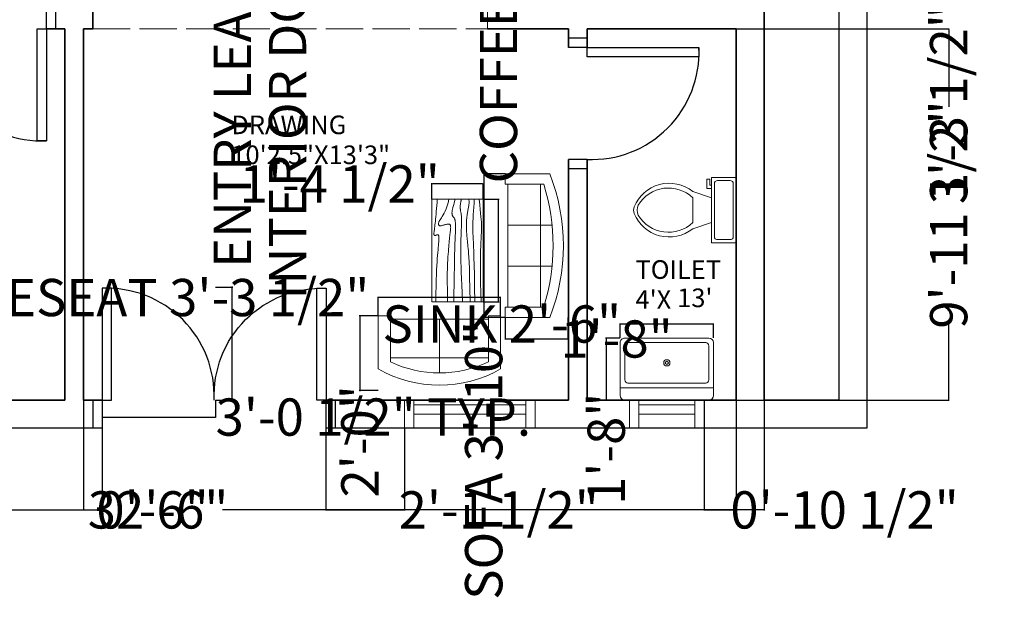
# Model space of a CAD drawing. Units: inches. Extents: x -107 to 531, y -526 to 131.
# Tile 2 of 4: x 205 to 522, y -526 to -340. Entities that reach past the tile are written whole.
import ezdxf

# ---------------------------------------------------------------- set-up
doc = ezdxf.new("R2010")
doc.units = ezdxf.units.IN
doc.header["$MEASUREMENT"] = 0
doc.linetypes.add('ACAD_ISO02W100', pattern=[15, 12, -3])
for name, color, linetype, lineweight in [('A-ANNO-DIMS', 2, 'Continuous', 18), ('A-AREA-IDEN', 7, 'Continuous', 25), ('A-DOOR', 3, 'Continuous', 25), ('A-FLOR-FIXT', 9, 'Continuous', 18), ('A-FLOR-STRS', 7, 'Continuous', 20), ('A-FURN', 8, 'Continuous', 18), ('A-GLAZ', 4, 'Continuous', 18), ('A-WALL', 7, 'Continuous', 35), ('A-WALL-OVHD', 8, 'ACAD_ISO02W100', 18), ('C-PROP', 8, 'Continuous', 25)]:
    doc.layers.add(name, color=color, linetype=linetype, lineweight=lineweight)
doc.styles.get("Standard").update_dxf_attribs({"font": 'arial.ttf'})
doc.dimstyles.get("Standard").update_dxf_attribs({"dimtxt": 12, "dimasz": 0.18, "dimexe": 0.18, "dimexo": 0.0625, "dimgap": 0.09, "dimtad": 0, "dimdec": 1, "dimzin": 0, "dimdsep": 46, "dimlunit": 3, "dimtxsty": 'Standard', "dimcen": 0.09, "dimadec": 0, "dimazin": 0, "dimtfac": 1, "dimtdec": 1, "dimtofl": 0, "dimtmove": 0, "dimatfit": 3, "dimfxl": 1, "dimtolj": 1, "dimtzin": 0, "dimarcsym": 0})

# ---------------------------------------------------------------- blocks, each defined once
blk = doc.blocks.new('Sofa - Roundback 7 ft.')
for p, q in [((-36.000027, -34), (-36.000027, -11.4696)), ((-12.00002, -32.4421), (-12.00003, -6.5971)), ((11.99997, -32.4421), (11.99998, -6.5971)), ((35.99998, -34), (35.99998, -11.4696)), ((-35.999844, -13.3819), (35.9998, -13.3819)), ((-36.000027, -32.4421), (35.99998, -32.4421))]:
    blk.add_line(p, q)
for points in [[(-36.000027, -34), (-42.000027, -34), (-42.000027, -8)], [(41.99998, -8), (41.99998, -34), (35.99998, -34)]]:
    blk.add_lwpolyline(points)
for centre, radius, start, end in [((0, -114.25), 114.25, 68.43141, 111.5686), ((-0.00001, -127.1968), 121.1968, 72.72033, 107.2797)]:
    blk.add_arc(centre, radius, start, end)
blk = doc.blocks.new('Sofa - Roundback Loveseat 5 ft.')
for p, q in [((0, -32.44198), (0, -5.99998)), ((-24, -33.99998), (-24, -11.46958)), ((-23.9998, -13.38178), (23.99986, -13.38178)), ((24.00004, -33.99998), (24.00004, -11.46958)), ((-24, -32.44198), (24.00004, -32.44198))]:
    blk.add_line(p, q)
for points in [[(-24, -33.99998), (-30, -33.99998), (-30, -7.99998)], [(30.00004, -7.99998), (30.00004, -33.99998), (24.00004, -33.99998)]]:
    blk.add_lwpolyline(points)
for centre, radius, start, end in [((0, -60.24998), 60.24998, 60.13715, 119.8628), ((0, -61.38438), 55.38444, 64.32083, 115.6792)]:
    blk.add_arc(centre, radius, start, end)
blk = doc.blocks.new('Table - Rectangular Woodgrain 60 x 30 in.')
for p, q in [((0, 0), (0, -30)), ((60, 0), (0, 0)), ((60, -30), (60, 0)), ((0, -30), (60, -30))]:
    blk.add_line(p, q)
for points in [[(0, -2.4), (4.8155, -2.418), (9.0302, -2.4688), (12.709, -2.5477), (15.9167, -2.65), (18.7181, -2.7711), (21.1781, -2.9063), (23.3616, -3.0508), (25.3333, -3.2), (27.1477, -3.3495), (28.8172, -3.4958), (30.3437, -3.636), (31.7291, -3.7667), (32.9756, -3.8849), (34.0849, -3.9875), (35.059, -4.0714), (35.9, -4.1334), (36.6114, -4.1711), (37.2041, -4.1854), (37.6906, -4.1779), (38.0833, -4.15), (38.3948, -4.1034), (38.6375, -4.0396), (38.8239, -3.9602), (38.9666, -3.8667), (39.0764, -3.7608), (39.1573, -3.6448), (39.2116, -3.521), (39.2416, -3.3917), (39.2498, -3.2593), (39.2385, -3.1261), (39.21, -2.9944), (39.1666, -2.8667), (39.111, -2.7447), (39.0468, -2.6281), (38.978, -2.5163), (38.9083, -2.4083), (38.8418, -2.3035), (38.7823, -2.201), (38.7337, -2.1001), (38.7, -2), (38.6844, -1.9003), (38.6875, -1.8021), (38.7094, -1.707), (38.75, -1.6167), (38.8094, -1.5326), (38.8875, -1.4563), (38.9844, -1.3893), (39.1, -1.3333), (39.2351, -1.2896), (39.3937, -1.2583), (39.5804, -1.2396), (39.8, -1.2333), (40.057, -1.2396), (40.3562, -1.2583), (40.7023, -1.2896), (41.1, -1.3333), (41.5547, -1.3895), (42.0755, -1.4573), (42.6721, -1.5361), (43.3542, -1.625), (44.1316, -1.7233), (45.014, -1.8302), (46.0114, -1.9449), (47.1333, -2.0667), (48.3862, -2.1947), (49.7625, -2.3281), (51.2513, -2.4663), (52.8416, -2.6083), (54.5226, -2.7535), (56.2833, -2.9011), (58.1127, -3.0501), (60, -3.2)], [(0, -9.2), (6.5759, -9.0858), (11.9385, -9.0365), (16.2527, -9.0418), (19.6833, -9.0917), (22.3952, -9.1759), (24.5531, -9.2844), (26.322, -9.4069), (27.8666, -9.5333), (29.3241, -9.6553), (30.7203, -9.7719), (32.0532, -9.8837), (33.3208, -9.9917), (34.5213, -10.0965), (35.6526, -10.199), (36.7128, -10.2999), (37.7, -10.4), (38.6129, -10.4996), (39.4531, -10.5969), (40.223, -10.6895), (40.925, -10.775), (41.5613, -10.8512), (42.1344, -10.9156), (42.6465, -10.966), (43.1, -11), (43.4976, -11.0158), (43.8437, -11.0136), (44.143, -10.9942), (44.4, -10.9583), (44.6195, -10.9069), (44.8062, -10.8406), (44.9648, -10.7603), (45.1, -10.6667), (45.2155, -10.5598), (45.3114, -10.4365), (45.3871, -10.2929), (45.4416, -10.125), (45.4743, -9.929), (45.4844, -9.7011), (45.4709, -9.4371), (45.4333, -9.1333), (45.3716, -8.7883), (45.2896, -8.4104), (45.1919, -8.0107), (45.0833, -7.6), (44.9685, -7.1893), (44.8521, -6.7896), (44.7388, -6.4117), (44.6333, -6.0667), (44.54, -5.7628), (44.4614, -5.4979), (44.4001, -5.2675), (44.3583, -5.0667), (44.3384, -4.8909), (44.3427, -4.7354), (44.3736, -4.5956), (44.4333, -4.4667), (44.5236, -4.3453), (44.6427, -4.2333), (44.7884, -4.1339), (44.9583, -4.05), (45.1501, -3.9849), (45.3614, -3.9417), (45.59, -3.9234), (45.8333, -3.9333), (46.0915, -3.9749), (46.3734, -4.0531), (46.6906, -4.1736), (47.0542, -4.3417), (47.4756, -4.5629), (47.9661, -4.8427), (48.5372, -5.1866), (49.2, -5.6), (49.9676, -6.0844), (50.8594, -6.625), (51.8965, -7.2031), (53.1, -7.8), (54.491, -8.3969), (56.0906, -8.975), (57.9199, -9.5156), (60, -10)], [(0, -12.8), (5.1847, -12.9322), (9.6213, -13.0323), (13.3963, -13.1059), (16.5958, -13.1583), (19.3063, -13.1952), (21.614, -13.2219), (23.6054, -13.2439), (25.3666, -13.2667), (26.9728, -13.2947), (28.4531, -13.3281), (29.8256, -13.3663), (31.1083, -13.4083), (32.3191, -13.4535), (33.476, -13.501), (34.597, -13.5501), (35.7, -13.6), (36.7984, -13.6497), (37.8875, -13.6979), (38.9578, -13.743), (40, -13.7833), (41.0047, -13.8174), (41.9625, -13.8438), (42.864, -13.8607), (43.7, -13.8667), (44.4631, -13.8604), (45.1552, -13.8417), (45.7801, -13.8104), (46.3416, -13.7667), (46.8439, -13.7104), (47.2906, -13.6417), (47.6858, -13.5604), (48.0333, -13.4667), (48.3375, -13.3608), (48.6042, -13.2448), (48.8396, -13.121), (49.05, -12.9917), (49.2417, -12.8593), (49.4208, -12.7261), (49.5937, -12.5944), (49.7667, -12.4667), (49.9452, -12.3451), (50.1323, -12.2313), (50.3303, -12.1268), (50.5416, -12.0333), (50.7686, -11.9524), (51.0135, -11.8854), (51.2788, -11.8341), (51.5666, -11.8), (51.8785, -11.7843), (52.2116, -11.7865), (52.562, -11.8059), (52.926, -11.8417), (53.2998, -11.8931), (53.6795, -11.9594), (54.0614, -12.0397), (54.4416, -12.1333), (54.8223, -12.2401), (55.2293, -12.3625), (55.6942, -12.5037), (56.2489, -12.6667), (56.9251, -12.8547), (57.7545, -13.0708), (58.7689, -13.3182), (60, -13.6)], [(0, -18), (5.124, -17.7273), (9.6609, -17.5057), (13.6705, -17.3303), (17.2125, -17.1958), (20.3467, -17.0973), (23.1328, -17.0297), (25.6307, -16.9878), (27.9, -16.9667), (29.9928, -16.9617), (31.9302, -16.9703), (33.7254, -16.9907), (35.3917, -17.0208), (36.9423, -17.0588), (38.3906, -17.1026), (39.7499, -17.1503), (41.0333, -17.2), (42.2519, -17.2496), (43.4073, -17.2969), (44.4986, -17.3395), (45.525, -17.375), (46.4858, -17.4012), (47.3802, -17.4156), (48.2074, -17.416), (48.9667, -17.4), (49.6583, -17.3662), (50.2872, -17.3167), (50.8595, -17.2547), (51.3812, -17.1833), (51.8584, -17.1057), (52.2971, -17.025), (52.7034, -16.9443), (53.0833, -16.8667), (53.443, -16.7951), (53.789, -16.7313), (54.128, -16.6768), (54.4666, -16.6334), (54.8115, -16.6024), (55.1693, -16.5854), (55.5465, -16.5841), (55.95, -16.6), (56.3828, -16.6337), (56.8346, -16.6823), (57.2915, -16.7418), (57.7396, -16.8084), (58.165, -16.878), (58.5539, -16.9469), (58.8924, -17.0111), (59.1666, -17.0667), (59.3679, -17.1107), (59.5078, -17.1438), (59.6032, -17.1675), (59.6708, -17.1833), (59.7275, -17.193), (59.7901, -17.1979), (59.8753, -17.1998), (60, -17.2)], [(0, -22.4), (8.0098, -22.2501), (14.4094, -22.1011), (19.4168, -21.9535), (23.25, -21.8083), (26.1269, -21.6663), (28.2656, -21.5281), (29.884, -21.3947), (31.2, -21.2667), (32.3967, -21.1448), (33.5172, -21.0292), (34.5697, -20.9198), (35.5625, -20.8167), (36.5037, -20.7198), (37.4015, -20.6292), (38.2642, -20.5448), (39.1, -20.4667), (39.9164, -20.3951), (40.7187, -20.3313), (41.5117, -20.2768), (42.3, -20.2333), (43.0883, -20.2024), (43.8812, -20.1854), (44.6836, -20.1841), (45.5, -20.2), (46.3328, -20.234), (47.1747, -20.2844), (48.0163, -20.3488), (48.8479, -20.425), (49.66, -20.5106), (50.4429, -20.6031), (51.1872, -20.7004), (51.8833, -20.8), (52.5246, -20.8999), (53.1166, -20.9995), (53.6681, -21.0983), (54.1875, -21.1958), (54.6834, -21.2919), (55.1646, -21.3859), (55.6394, -21.4777), (56.1167, -21.5667), (56.6028, -21.6515), (57.0961, -21.7266), (57.5929, -21.7852), (58.0896, -21.8208), (58.5823, -21.8268), (59.0674, -21.7964), (59.5412, -21.723), (60, -21.6)], [(0, -25.2), (8.6355, -25.0504), (15.7026, -24.9031), (21.4049, -24.7606), (25.9458, -24.625), (29.529, -24.4988), (32.3578, -24.3844), (34.6359, -24.284), (36.5667, -24.2), (38.3213, -24.1341), (39.9417, -24.0854), (41.437, -24.0523), (42.8167, -24.0333), (44.0901, -24.0268), (45.2667, -24.0313), (46.3557, -24.0451), (47.3667, -24.0667), (48.309, -24.0947), (49.1928, -24.1287), (50.0284, -24.168), (50.826, -24.2125), (51.5959, -24.2617), (52.3483, -24.3151), (53.0935, -24.3725), (53.8417, -24.4334), (54.6009, -24.497), (55.3699, -24.561), (56.1454, -24.6226), (56.9239, -24.6792), (57.7021, -24.7279), (58.4764, -24.7662), (59.2435, -24.7911), (60, -24.8)], [(0, -28.8), (5.6867, -28.6681), (10.45, -28.5698), (14.407, -28.5012), (17.675, -28.4584), (20.3711, -28.4374), (22.6125, -28.4344), (24.5164, -28.4455), (26.2, -28.4667), (27.762, -28.4947), (29.2276, -28.5281), (30.6033, -28.5663), (31.8958, -28.6084), (33.1118, -28.6535), (34.2578, -28.7011), (35.3405, -28.7501), (36.3666, -28.8), (37.3443, -28.8497), (38.288, -28.8974), (39.2137, -28.9412), (40.1375, -28.9792), (41.0753, -29.0093), (42.0432, -29.0297), (43.0572, -29.0384), (44.1333, -29.0333), (45.2936, -29.0114), (46.5843, -28.9641), (48.0579, -28.8816), (49.7666, -28.7542), (51.7629, -28.5721), (54.0989, -28.3255), (56.8272, -28.0048), (60, -27.6)]]:
    blk.add_lwpolyline(points)
blk = doc.blocks.new('Toilet - top')
for p, q in [((9.5, -6), (9.5, -2)), ((-10, -8.5), (-8, -8.5)), ((-10, -9.5), (-10, -8.5)), ((-7, -9.5), (-10, -9.5)), ((-8, -8.5), (-8, -8)), ((-7, -8), (-7, -9.5)), ((-4, -8), (-6, -14)), ((4, -8), (6, -14)), ((4, -14), (-4, -14))]:
    blk.add_line(p, q)
blk.add_lwpolyline([(10.5, -8), (10.5, 0), (-10.5, 0), (-10.5, -8)], close=True)
for points in [[(-9.5, -2), (-9.5, -6)], [(8.5, -1), (-8.5, -1)], [(-8.5, -7), (8.5, -7)]]:
    blk.add_lwpolyline(points)
for centre, radius, start, end in [((-8.62, -1.88), 0.884, 81.8699, 188.1301), ((8.62, -1.88), 0.884, 351.8699, 98.1301), ((-8.62, -6.12), 0.884, 171.8699, 278.1301), ((8.62, -6.12), 0.884, 261.8699, 8.1301), ((3.52, -21.58), 12.17, 141.4691, 247.9714), ((4.2, -21.82), 11.33, 136.3677, 238.9468), ((-3.52, -21.58), 12.17, 292.0284, 38.5307), ((-4.2, -21.82), 11.33, 301.053, 43.6321), ((0, -27.88), 4, 245.7318, 294.2682), ((0, -29), 4, 254.8605, 285.1395)]:
    blk.add_arc(centre, radius, start, end)
blk = doc.blocks.new('Sink-single - 30 in top')
blk.add_line((-15, -3.999996), (15, -3.999996))
for points in [[(-13.5, 0), (13.5, 0)], [(-15, -18.499996), (-15, -1.5)], [(15, -1.5), (15, -18.499996)], [(-12.5, -5.499996), (12.5, -5.499996)], [(-13.5, -17.499996), (-13.5, -6.499996)], [(13.5, -6.499996), (13.5, -17.499996)], [(12.5, -18.499996), (-12.5, -18.499996)], [(13.5, -19.999996), (-13.5, -19.999996)]]:
    blk.add_lwpolyline(points)
for radius in [1, 0.5]:
    blk.add_circle((0, -11.999996), radius)
for centre, radius, start, end in [((-13.5, -1.5), 1.5, 90, 180), ((13.5, -1.5), 1.5, 0, 90), ((-12.5, -6.499996), 1, 90, 180), ((12.5, -6.499996), 1, 0, 90), ((-13.5, -18.499996), 1.5, 180, 270), ((-12.5, -17.499996), 1, 180, 270), ((12.5, -17.499996), 1, 270, 0), ((13.5, -18.499996), 1.5, 270, 0)]:
    blk.add_arc(centre, radius, start, end)
blk = doc.blocks.new('WIN-36')
for p, q in [((0, 0), (0, 9)), ((3, 0), (3, 9)), ((3, 9), (39, 9)), ((39, 7.5), (3, 7.5)), ((39, 9), (39, 0)), ((42, 9), (42, 0)), ((39, 4.5), (3, 4.5)), ((39, 0), (3, 0))]:
    blk.add_line(p, q)
blk = doc.blocks.new('WIN-18')
for p, q in [((0, 9), (0, 0)), ((21, 9), (3, 9)), ((3, 9), (3, 0)), ((21, 0), (21, 9)), ((24, 0), (24, 9)), ((3, 4.5), (21, 4.5)), ((3, 1.5), (21, 1.5)), ((3, 0), (21, 0))]:
    blk.add_line(p, q)
blk = doc.blocks.new('DOOR-36-SWING')
for p, q in [((36.03, 42), (42.03, 42)), ((36.03, 39), (42.03, 39)), ((36.03, 3), (42.03, 3)), ((36.03, 0), (42.03, 0))]:
    blk.add_line(p, q)
blk.add_lwpolyline([(36.03, 3), (0.03, 3), (0.03, 6), (36.03, 6)], close=True)
blk.add_arc((34.53, 4.5), 34.53, 87.5104, 182.4896)
blk = doc.blocks.new('ENTRY-LEAF-36')
blk.add_lwpolyline([(0, 0), (3, 0), (3, 36), (0, 36)], close=True)
blk.add_arc((1.5, 1.5), 34.53, 357.5104, 92.4896)
blk = doc.blocks.new('*D27')
at = {"layer": 'A-ANNO-DIMS', "color": 0, "lineweight": -2, "transparency": 16777216}
for p, q in [((268.43, -425.94), (274.01, -425.94)), ((273.83, -425.94), (273.83, -425.76)), ((273.83, -462.18), (273.83, -426.12)), ((268.43, -462.36), (274.01, -462.36))]:
    blk.add_line(p, q, dxfattribs=at)
at = {"layer": 'A-ANNO-DIMS', "color": 0, "transparency": 16777216}
for points in [[(273.8, -426.12), (273.86, -426.12), (273.83, -425.94)], [(273.8, -462.18), (273.86, -462.18), (273.83, -462.36)]]:
    blk.add_solid(points, dxfattribs=at)
at = {"layer": 'Defpoints', "color": 0, "transparency": 16777216}
for p in [(268.37, -425.94), (273.83, -425.94), (268.37, -462.36)]:
    blk.add_point(p, dxfattribs=at)
at = {"layer": 'A-ANNO-DIMS', "color": 0, "transparency": 16777216, "insert": (273.83, -321.4), "char_height": 12, "attachment_point": 5, "rotation": 90}
blk.add_mtext('\\A1;ENTRY LEAF 3\'-0 1/2" TYP.', dxfattribs=at)
blk = doc.blocks.new('*D28')
at = {"layer": 'A-ANNO-DIMS', "color": 0, "lineweight": -2, "transparency": 16777216}
for p, q in [((231.95, -462.42), (231.95, -468)), ((268.37, -462.42), (268.37, -468)), ((232.13, -467.82), (268.19, -467.82)), ((268.37, -467.82), (268.55, -467.82))]:
    blk.add_line(p, q, dxfattribs=at)
at = {"layer": 'A-ANNO-DIMS', "color": 0, "transparency": 16777216}
for points in [[(232.13, -467.79), (232.13, -467.85), (231.95, -467.82)], [(268.19, -467.79), (268.19, -467.85), (268.37, -467.82)]]:
    blk.add_solid(points, dxfattribs=at)
at = {"layer": 'Defpoints', "color": 0, "transparency": 16777216}
for p in [(231.95, -462.36), (268.37, -462.36), (268.37, -467.82)]:
    blk.add_point(p, dxfattribs=at)
at = {"layer": 'A-ANNO-DIMS', "color": 0, "transparency": 16777216, "insert": (319.19, -467.82), "char_height": 12, "attachment_point": 5}
blk.add_mtext('\\A1;3\'-0 1/2" TYP.', dxfattribs=at)
blk = doc.blocks.new('*D29')
at = {"layer": 'A-ANNO-DIMS', "color": 0, "lineweight": -2, "transparency": 16777216}
for p, q in [((297.89, -152.94), (291.41, -152.94)), ((291.59, -153.12), (291.59, -195.18)), ((297.89, -195.36), (291.41, -195.36)), ((291.59, -195.36), (291.59, -195.54))]:
    blk.add_line(p, q, dxfattribs=at)
at = {"layer": 'A-ANNO-DIMS', "color": 0, "transparency": 16777216}
for points in [[(291.56, -153.12), (291.62, -153.12), (291.59, -152.94)], [(291.56, -195.18), (291.62, -195.18), (291.59, -195.36)]]:
    blk.add_solid(points, dxfattribs=at)
at = {"layer": 'Defpoints', "color": 0, "transparency": 16777216}
for p in [(297.95, -152.94), (291.59, -195.36), (297.95, -195.36)]:
    blk.add_point(p, dxfattribs=at)
at = {"layer": 'A-ANNO-DIMS', "color": 0, "transparency": 16777216, "insert": (291.59, -315.6), "char_height": 12, "attachment_point": 5, "rotation": 90}
blk.add_mtext('\\A1;INTERIOR DOOR 3\'-6 1/2" TYP.', dxfattribs=at)
blk = doc.blocks.new('*D37')
at = {"layer": 'A-ANNO-DIMS', "color": 0, "lineweight": -2, "transparency": 16777216}
for p, q in [((398.62, -437.86), (398.44, -437.86)), ((398.62, -442.3), (398.62, -437.68)), ((428.44, -437.86), (398.8, -437.86)), ((428.62, -442.3), (428.62, -437.68))]:
    blk.add_line(p, q, dxfattribs=at)
at = {"layer": 'A-ANNO-DIMS', "color": 0, "transparency": 16777216}
for points in [[(398.8, -437.83), (398.8, -437.89), (398.62, -437.86)], [(428.44, -437.83), (428.44, -437.89), (428.62, -437.86)]]:
    blk.add_solid(points, dxfattribs=at)
at = {"layer": 'Defpoints', "color": 0, "transparency": 16777216}
for p in [(398.62, -437.86), (398.62, -442.36), (428.62, -442.36)]:
    blk.add_point(p, dxfattribs=at)
at = {"layer": 'A-ANNO-DIMS', "color": 0, "transparency": 16777216, "insert": (360.53, -437.86), "char_height": 12, "attachment_point": 5}
blk.add_mtext('\\A1;SINK 2\'-6"', dxfattribs=at)
blk = doc.blocks.new('*D38')
at = {"layer": 'A-ANNO-DIMS', "color": 0, "lineweight": -2, "transparency": 16777216}
for p, q in [((398.55, -442.36), (393.94, -442.36)), ((394.12, -442.54), (394.12, -462.18)), ((398.55, -462.36), (393.94, -462.36)), ((394.12, -462.36), (394.12, -462.54))]:
    blk.add_line(p, q, dxfattribs=at)
at = {"layer": 'A-ANNO-DIMS', "color": 0, "transparency": 16777216}
for points in [[(394.09, -442.54), (394.15, -442.54), (394.12, -442.36)], [(394.09, -462.18), (394.15, -462.18), (394.12, -462.36)]]:
    blk.add_solid(points, dxfattribs=at)
at = {"layer": 'Defpoints', "color": 0, "transparency": 16777216}
for p in [(398.62, -442.36), (394.12, -462.36), (398.62, -462.36)]:
    blk.add_point(p, dxfattribs=at)
at = {"layer": 'A-ANNO-DIMS', "color": 0, "transparency": 16777216, "insert": (394.12, -478.02), "char_height": 12, "attachment_point": 5, "rotation": 90}
blk.add_mtext('\\A1;1\'-8"', dxfattribs=at)
blk = doc.blocks.new('*D45')
at = {"layer": 'A-ANNO-DIMS', "color": 0, "lineweight": -2, "transparency": 16777216}
for p, q in [((361.57, -389.52), (354.52, -389.52)), ((354.7, -389.7), (354.7, -435.56)), ((361.57, -435.74), (354.52, -435.74)), ((354.7, -435.74), (354.7, -435.92))]:
    blk.add_line(p, q, dxfattribs=at)
at = {"layer": 'A-ANNO-DIMS', "color": 0, "transparency": 16777216}
for points in [[(354.67, -389.7), (354.73, -389.7), (354.7, -389.52)], [(354.67, -435.56), (354.73, -435.56), (354.7, -435.74)]]:
    blk.add_solid(points, dxfattribs=at)
at = {"layer": 'Defpoints', "color": 0, "transparency": 16777216}
for p in [(361.63, -389.52), (354.7, -435.74), (361.63, -435.74)]:
    blk.add_point(p, dxfattribs=at)
at = {"layer": 'A-ANNO-DIMS', "color": 0, "transparency": 16777216, "insert": (354.7, -481.74), "char_height": 12, "attachment_point": 5, "rotation": 90}
blk.add_mtext('\\A1;SOFA 3\'-10"', dxfattribs=at)
blk = doc.blocks.new('*D46')
at = {"layer": 'A-ANNO-DIMS', "color": 0, "lineweight": -2, "transparency": 16777216}
for p, q in [((361.63, -435.8), (361.63, -442.85)), ((381.81, -435.8), (381.81, -442.85)), ((361.81, -442.67), (381.63, -442.67)), ((381.81, -442.67), (381.99, -442.67))]:
    blk.add_line(p, q, dxfattribs=at)
at = {"layer": 'A-ANNO-DIMS', "color": 0, "transparency": 16777216}
for points in [[(361.81, -442.64), (361.81, -442.7), (361.63, -442.67)], [(381.63, -442.64), (381.63, -442.7), (381.81, -442.67)]]:
    blk.add_solid(points, dxfattribs=at)
at = {"layer": 'Defpoints', "color": 0, "transparency": 16777216}
for p in [(361.63, -435.74), (381.81, -435.74), (381.81, -442.67)]:
    blk.add_point(p, dxfattribs=at)
at = {"layer": 'A-ANNO-DIMS', "color": 0, "transparency": 16777216, "insert": (397.46, -442.67), "char_height": 12, "attachment_point": 5}
blk.add_mtext('\\A1;1\'-8"', dxfattribs=at)
blk = doc.blocks.new('*D47')
at = {"layer": 'A-ANNO-DIMS', "color": 0, "lineweight": -2, "transparency": 16777216}
for p, q in [((320.77, -429.33), (320.59, -429.33)), ((320.77, -435.18), (320.77, -429.15)), ((359.96, -429.33), (320.95, -429.33)), ((360.14, -435.18), (360.14, -429.15))]:
    blk.add_line(p, q, dxfattribs=at)
at = {"layer": 'A-ANNO-DIMS', "color": 0, "transparency": 16777216}
for points in [[(320.95, -429.3), (320.95, -429.36), (320.77, -429.33)], [(359.96, -429.3), (359.96, -429.36), (360.14, -429.33)]]:
    blk.add_solid(points, dxfattribs=at)
at = {"layer": 'Defpoints', "color": 0, "transparency": 16777216}
for p in [(320.77, -429.33), (320.77, -435.24), (360.14, -435.24)]:
    blk.add_point(p, dxfattribs=at)
at = {"layer": 'A-ANNO-DIMS', "color": 0, "transparency": 16777216, "insert": (244.25, -429.33), "char_height": 12, "attachment_point": 5}
blk.add_mtext('\\A1;LOVESEAT 3\'-3 1/2"', dxfattribs=at)
blk = doc.blocks.new('*D48')
at = {"layer": 'A-ANNO-DIMS', "color": 0, "lineweight": -2, "transparency": 16777216}
for p, q in [((320.71, -435.24), (314.69, -435.24)), ((314.87, -435.42), (314.87, -459.12)), ((320.71, -459.3), (314.69, -459.3)), ((314.87, -459.3), (314.87, -459.48))]:
    blk.add_line(p, q, dxfattribs=at)
at = {"layer": 'A-ANNO-DIMS', "color": 0, "transparency": 16777216}
for points in [[(314.84, -435.42), (314.9, -435.42), (314.87, -435.24)], [(314.84, -459.12), (314.9, -459.12), (314.87, -459.3)]]:
    blk.add_solid(points, dxfattribs=at)
at = {"layer": 'Defpoints', "color": 0, "transparency": 16777216}
for p in [(320.77, -435.24), (314.87, -459.3), (320.77, -459.3)]:
    blk.add_point(p, dxfattribs=at)
at = {"layer": 'A-ANNO-DIMS', "color": 0, "transparency": 16777216, "insert": (314.87, -475.62), "char_height": 12, "attachment_point": 5, "rotation": 90}
blk.add_mtext('\\A1;2\'-0"', dxfattribs=at)
blk = doc.blocks.new('*D49')
at = {"layer": 'A-ANNO-DIMS', "color": 0, "lineweight": -2, "transparency": 16777216}
for p, q in [((354.58, -397.68), (359.64, -397.68)), ((359.46, -397.68), (359.46, -397.5)), ((359.46, -430.49), (359.46, -397.86)), ((354.58, -430.67), (359.64, -430.67))]:
    blk.add_line(p, q, dxfattribs=at)
at = {"layer": 'A-ANNO-DIMS', "color": 0, "transparency": 16777216}
for points in [[(359.43, -397.86), (359.49, -397.86), (359.46, -397.68)], [(359.43, -430.49), (359.49, -430.49), (359.46, -430.67)]]:
    blk.add_solid(points, dxfattribs=at)
at = {"layer": 'Defpoints', "color": 0, "transparency": 16777216}
for p in [(354.51, -397.68), (359.46, -397.68), (354.51, -430.67)]:
    blk.add_point(p, dxfattribs=at)
at = {"layer": 'A-ANNO-DIMS', "color": 0, "transparency": 16777216, "insert": (359.46, -316.33), "char_height": 12, "attachment_point": 5, "rotation": 90}
blk.add_mtext('\\A1;COFFEE TABLE 2\'-9"', dxfattribs=at)
blk = doc.blocks.new('*D50')
at = {"layer": 'A-ANNO-DIMS', "color": 0, "lineweight": -2, "transparency": 16777216}
for p, q in [((338.02, -392.74), (337.84, -392.74)), ((338.02, -397.62), (338.02, -392.56)), ((354.33, -392.74), (338.2, -392.74)), ((354.51, -397.62), (354.51, -392.56))]:
    blk.add_line(p, q, dxfattribs=at)
at = {"layer": 'A-ANNO-DIMS', "color": 0, "transparency": 16777216}
for points in [[(338.2, -392.71), (338.2, -392.77), (338.02, -392.74)], [(354.33, -392.71), (354.33, -392.77), (354.51, -392.74)]]:
    blk.add_solid(points, dxfattribs=at)
at = {"layer": 'Defpoints', "color": 0, "transparency": 16777216}
for p in [(338.02, -392.74), (338.02, -397.68), (354.51, -397.68)]:
    blk.add_point(p, dxfattribs=at)
at = {"layer": 'A-ANNO-DIMS', "color": 0, "transparency": 16777216, "insert": (308.39, -392.74), "char_height": 12, "attachment_point": 5}
blk.add_mtext('\\A1;1\'-4 1/2"', dxfattribs=at)
blk = doc.blocks.new('*D59')
at = {"layer": 'A-ANNO-DIMS', "color": 0, "lineweight": -2, "transparency": 16777216}
for p, q in [((54.95, -462.42), (54.95, -497.89)), ((444.95, -462.42), (444.95, -497.89)), ((55.13, -497.71), (229.25, -497.71)), ((444.77, -497.71), (270.65, -497.71))]:
    blk.add_line(p, q, dxfattribs=at)
at = {"layer": 'A-ANNO-DIMS', "color": 0, "transparency": 16777216}
for points in [[(55.13, -497.68), (55.13, -497.74), (54.95, -497.71)], [(444.77, -497.68), (444.77, -497.74), (444.95, -497.71)]]:
    blk.add_solid(points, dxfattribs=at)
at = {"layer": 'Defpoints', "color": 0, "transparency": 16777216}
for p in [(54.95, -462.36), (444.95, -462.36), (444.95, -497.71)]:
    blk.add_point(p, dxfattribs=at)
at = {"layer": 'A-ANNO-DIMS', "color": 0, "transparency": 16777216, "insert": (249.95, -497.71), "char_height": 12, "attachment_point": 5}
blk.add_mtext('\\A1;32\'-6"', dxfattribs=at)
blk = doc.blocks.new('*D61')
at = {"layer": 'A-ANNO-DIMS', "color": 0, "lineweight": -2, "transparency": 16777216}
for p, q in [((436.01, -297.36), (504.48, -297.36)), ((504.3, -297.54), (504.3, -336.68)), ((436.01, -336.86), (504.48, -336.86)), ((504.3, -336.86), (504.3, -337.04))]:
    blk.add_line(p, q, dxfattribs=at)
at = {"layer": 'A-ANNO-DIMS', "color": 0, "transparency": 16777216}
for points in [[(504.27, -297.54), (504.33, -297.54), (504.3, -297.36)], [(504.27, -336.68), (504.33, -336.68), (504.3, -336.86)]]:
    blk.add_solid(points, dxfattribs=at)
at = {"layer": 'Defpoints', "color": 0, "transparency": 16777216}
for p in [(435.95, -297.36), (435.95, -336.86), (504.3, -336.86)]:
    blk.add_point(p, dxfattribs=at)
at = {"layer": 'A-ANNO-DIMS', "color": 0, "transparency": 16777216, "insert": (504.3, -367.06), "char_height": 12, "attachment_point": 5, "rotation": 90}
blk.add_mtext('\\A1;3\'-3 1/2"', dxfattribs=at)
blk = doc.blocks.new('*D66')
at = {"layer": 'A-ANNO-DIMS', "color": 0, "lineweight": -2, "transparency": 16777216}
for p, q in [((225.95, -462.42), (225.95, -497.89)), ((231.95, -462.42), (231.95, -497.89)), ((226.13, -497.71), (231.77, -497.71)), ((231.95, -497.71), (232.13, -497.71))]:
    blk.add_line(p, q, dxfattribs=at)
at = {"layer": 'A-ANNO-DIMS', "color": 0, "transparency": 16777216}
for points in [[(226.13, -497.68), (226.13, -497.74), (225.95, -497.71)], [(231.77, -497.68), (231.77, -497.74), (231.95, -497.71)]]:
    blk.add_solid(points, dxfattribs=at)
at = {"layer": 'Defpoints', "color": 0, "transparency": 16777216}
for p in [(225.95, -462.36), (231.95, -462.36), (231.95, -497.71)]:
    blk.add_point(p, dxfattribs=at)
at = {"layer": 'A-ANNO-DIMS', "color": 0, "transparency": 16777216, "insert": (248.17, -497.71), "char_height": 12, "attachment_point": 5}
blk.add_mtext('\\A1;0\'-6"', dxfattribs=at)
blk = doc.blocks.new('*D67')
at = {"layer": 'A-ANNO-DIMS', "color": 0, "lineweight": -2, "transparency": 16777216}
for p, q in [((303.95, -471.42), (303.95, -497.89)), ((329.25, -471.42), (329.25, -497.89)), ((304.13, -497.71), (329.07, -497.71)), ((329.25, -497.71), (329.43, -497.71))]:
    blk.add_line(p, q, dxfattribs=at)
at = {"layer": 'A-ANNO-DIMS', "color": 0, "transparency": 16777216}
for points in [[(304.13, -497.68), (304.13, -497.74), (303.95, -497.71)], [(329.07, -497.68), (329.07, -497.74), (329.25, -497.71)]]:
    blk.add_solid(points, dxfattribs=at)
at = {"layer": 'Defpoints', "color": 0, "transparency": 16777216}
for p in [(303.95, -471.36), (329.25, -471.36), (329.25, -497.71)]:
    blk.add_point(p, dxfattribs=at)
at = {"layer": 'A-ANNO-DIMS', "color": 0, "transparency": 16777216, "insert": (359.55, -497.71), "char_height": 12, "attachment_point": 5}
blk.add_mtext('\\A1;2\'-1 1/2"', dxfattribs=at)
blk = doc.blocks.new('*D68')
at = {"layer": 'A-ANNO-DIMS', "color": 0, "lineweight": -2, "transparency": 16777216}
for p, q in [((425.62, -462.42), (425.62, -497.89)), ((435.95, -462.42), (435.95, -497.89)), ((425.8, -497.71), (435.77, -497.71)), ((435.95, -497.71), (436.13, -497.71))]:
    blk.add_line(p, q, dxfattribs=at)
at = {"layer": 'A-ANNO-DIMS', "color": 0, "transparency": 16777216}
for points in [[(425.8, -497.68), (425.8, -497.74), (425.62, -497.71)], [(435.77, -497.68), (435.77, -497.74), (435.95, -497.71)]]:
    blk.add_solid(points, dxfattribs=at)
at = {"layer": 'Defpoints', "color": 0, "transparency": 16777216}
for p in [(425.62, -462.36), (435.95, -462.36), (435.95, -497.71)]:
    blk.add_point(p, dxfattribs=at)
at = {"layer": 'A-ANNO-DIMS', "color": 0, "transparency": 16777216, "insert": (470.81, -497.71), "char_height": 12, "attachment_point": 5}
blk.add_mtext('\\A1;0\'-10 1/2"', dxfattribs=at)
blk = doc.blocks.new('*D69')
at = {"layer": 'A-ANNO-DIMS', "color": 0, "lineweight": -2, "transparency": 16777216}
for p, q in [((436.01, -342.86), (504.48, -342.86)), ((504.3, -343.04), (504.3, -367.93)), ((504.3, -462.18), (504.3, -437.29)), ((436.01, -462.36), (504.48, -462.36))]:
    blk.add_line(p, q, dxfattribs=at)
at = {"layer": 'A-ANNO-DIMS', "color": 0, "transparency": 16777216}
for points in [[(504.27, -343.04), (504.33, -343.04), (504.3, -342.86)], [(504.27, -462.18), (504.33, -462.18), (504.3, -462.36)]]:
    blk.add_solid(points, dxfattribs=at)
at = {"layer": 'Defpoints', "color": 0, "transparency": 16777216}
for p in [(435.95, -342.86), (504.3, -342.86), (435.95, -462.36)]:
    blk.add_point(p, dxfattribs=at)
at = {"layer": 'A-ANNO-DIMS', "color": 0, "transparency": 16777216, "insert": (504.3, -402.61), "char_height": 12, "attachment_point": 5, "rotation": 90}
blk.add_mtext('\\A1;9\'-11 1/2"', dxfattribs=at)

msp = doc.modelspace()

# ---------------------------------------------------------------- linework, layer by layer
at = {"layer": 'A-DOOR'}
for p, q in [((228.95, -462.36), (231.95, -462.36)), ((231.95, -462.36), (228.95, -462.36)), ((228.95, -462.36), (228.95, -471.36)), ((231.95, -462.36), (231.95, -471.36)), ((303.95, -462.36), (303.95, -471.36)), ((306.95, -462.36), (306.95, -471.36))]:
    msp.add_line(p, q, dxfattribs=at)
at = {"layer": 'A-FLOR-STRS'}
msp.add_line((355.95, -297.36), (355.95, -342.86), dxfattribs=at)
at = {"layer": 'A-WALL'}
for p, q in [((444.95, -24.36), (444.95, -462.36)), ((228.95, -342.86), (228.95, -336.86)), ((214.07, -342.86), (219.95, -342.86)), ((219.95, -462.36), (219.95, -342.86)), ((225.95, -462.36), (225.95, -342.86)), ((225.95, -342.86), (228.95, -342.86)), ((355.95, -342.86), (381.95, -342.86)), ((381.95, -342.86), (381.95, -348.86)), ((387.95, -342.86), (387.95, -348.86)), ((387.95, -342.86), (435.95, -342.86)), ((435.95, -342.86), (435.95, -462.36)), ((381.95, -384.86), (381.95, -462.36)), ((387.95, -384.86), (387.95, -462.36)), ((219.95, -462.36), (63.95, -462.36)), ((231.95, -462.36), (225.95, -462.36)), ((381.95, -462.36), (303.95, -462.36)), ((435.95, -462.36), (387.95, -462.36))]:
    msp.add_line(p, q, dxfattribs=at)
at = {"layer": 'A-WALL-OVHD'}
msp.add_line((228.95, -342.86), (355.95, -342.86), dxfattribs=at)
at = {"layer": 'C-PROP'}
for p, q in [((468.95, -0.36), (468.95, -462.36)), ((468.95, -462.36), (444.95, -462.36))]:
    msp.add_line(p, q, dxfattribs=at)
msp.add_lwpolyline([(231.95, -471.36), (21.95, -471.36), (21.95, 8.64), (477.95, 8.64), (477.95, -471.36), (303.95, -471.36)], dxfattribs=at)

# ---------------------------------------------------------------- block references
at = {"layer": 'A-DOOR'}
for p, rotation in [((217.07, -378.89), 89.99999999999991), ((423.98, -345.86), 180)]:
    msp.add_blockref('DOOR-36-SWING', p, dxfattribs=dict(at, rotation=rotation))
msp.add_blockref('ENTRY-LEAF-36', (231.95, -462.36), dxfattribs=at)
at = {"layer": 'A-DOOR', "extrusion": (0, 0, -1), "zscale": -1}
msp.add_blockref('ENTRY-LEAF-36', (-304.02, -462.36), dxfattribs=at)
at = {"layer": 'A-FLOR-FIXT'}
for name, p, rotation in [('Toilet - top', (435.95, -401.19), 270), ('Sink-single - 30 in top', (413.62, -462.36), 180)]:
    msp.add_blockref(name, p, dxfattribs=dict(at, rotation=rotation))
at = {"layer": 'A-FURN'}
for name, p, xscale, yscale, zscale, rotation in [('Sofa - Roundback 7 ft.', (380.34, -412.63), 0.5502317276898082, 0.5502317276898082, 0.5502317276898082, 270), ('Table - Rectangular Woodgrain 60 x 30 in.', (338.02, -430.67), 0.5497164975129128, 0.5497164975129128, 0.5497164975129128, 90), ('Sofa - Roundback Loveseat 5 ft.', (340.46, -457.55), 0.656127879681973, 0.656127879681973, 0.656127879681973, 180)]:
    msp.add_blockref(name, p, dxfattribs=dict(at, xscale=xscale, yscale=yscale, zscale=zscale, rotation=rotation))
at = {"layer": 'A-GLAZ'}
msp.add_blockref('WIN-36', (329.25, -471.36), dxfattribs=at)
at = {"layer": 'A-GLAZ', "rotation": 180}
msp.add_blockref('WIN-18', (425.62, -462.36), dxfattribs=at)

# ---------------------------------------------------------------- texts
at = {"layer": 'A-AREA-IDEN'}
for s, p in [('DRAWING', (273.52, -376.73)), ('10\'2.5"X13\'3"', (273.52, -386.37)), ('TOILET', (403.53, -423.32)), ("4'X", (403.53, -432.96)), ("13'", (416.96, -432.43))]:
    msp.add_text(s, height=6, dxfattribs=at).set_placement(p)

# ---------------------------------------------------------------- dimensions: what is measured, and where the dimension line sits
at = {"layer": 'A-ANNO-DIMS'}
for base, p1, p2, angle, text, picture, middle in [((291.59, -195.36), (297.95, -152.94), (297.95, -195.36), 270, 'INTERIOR DOOR <> TYP.', '*D29', (291.59, -315.6)), ((273.83, -425.94), (268.37, -462.36), (268.37, -425.94), 90, 'ENTRY LEAF <> TYP.', '*D27', (273.83, -321.4)), ((359.46, -397.68), (354.51, -430.67), (354.51, -397.68), 90, 'COFFEE TABLE <>', '*D49', (359.46, -316.33)), ((354.7, -435.74), (361.63, -389.52), (361.63, -435.74), 270, 'SOFA <>', '*D45', (354.7, -481.74)), ((320.77, -429.33), (360.14, -435.24), (320.77, -435.24), 180, 'LOVESEAT <>', '*D47', (244.25, -429.33)), ((398.62, -437.86), (428.62, -442.36), (398.62, -442.36), 180, 'SINK <>', '*D37', (360.53, -437.86))]:
    dim = msp.add_linear_dim(base=base, p1=p1, p2=p2, angle=angle, text=text, dimstyle='Standard', override={"dimdec": 1, "dimlfac": 1, "dimrnd": 0, "dimzin": 1, "dimdsep": 46, "dimlunit": 4, "dimfrac": 2}, dxfattribs=at)
    dim.commit()
    dim.dimension.update_dxf_attribs({"geometry": picture, "text_midpoint": middle})
for base, p1, p2, angle, picture, middle in [((504.3, -336.86), (435.95, -297.36), (435.95, -336.86), 90, '*D61', (504.3, -367.06)), ((504.3, -342.86), (435.95, -462.36), (435.95, -342.86), 90, '*D69', (504.3, -402.61)), ((338.02, -392.74), (354.51, -397.68), (338.02, -397.68), 180, '*D50', (308.39, -392.74)), ((314.87, -459.3), (320.77, -435.24), (320.77, -459.3), 270, '*D48', (314.87, -475.62)), ((394.12, -462.36), (398.62, -442.36), (398.62, -462.36), 270, '*D38', (394.12, -478.02))]:
    dim = msp.add_linear_dim(base=base, p1=p1, p2=p2, angle=angle, dimstyle='Standard', override={"dimdec": 1, "dimlfac": 1, "dimrnd": 0, "dimzin": 1, "dimdsep": 46, "dimlunit": 4, "dimfrac": 2}, dxfattribs=at)
    dim.commit()
    dim.dimension.update_dxf_attribs({"geometry": picture, "text_midpoint": middle})
for base, p1, p2, picture, middle in [((381.81, -442.67), (361.63, -435.74), (381.81, -435.74), '*D46', (397.46, -442.67)), ((444.95, -497.71), (54.95, -462.36), (444.95, -462.36), '*D59', (249.95, -497.71)), ((231.95, -497.71), (225.95, -462.36), (231.95, -462.36), '*D66', (248.17, -497.71)), ((435.95, -497.71), (425.62, -462.36), (435.95, -462.36), '*D68', (470.81, -497.71)), ((329.25, -497.71), (303.95, -471.36), (329.25, -471.36), '*D67', (359.55, -497.71))]:
    dim = msp.add_linear_dim(base=base, p1=p1, p2=p2, dimstyle='Standard', override={"dimdec": 1, "dimlfac": 1, "dimrnd": 0, "dimzin": 1, "dimdsep": 46, "dimlunit": 4, "dimfrac": 2}, dxfattribs=at)
    dim.commit()
    dim.dimension.update_dxf_attribs({"geometry": picture, "text_midpoint": middle})
dim = msp.add_linear_dim(base=(268.37, -467.82), p1=(231.95, -462.36), p2=(268.37, -462.36), text='<> TYP.', dimstyle='Standard', override={"dimdec": 1, "dimlfac": 1, "dimrnd": 0, "dimzin": 1, "dimdsep": 46, "dimlunit": 4, "dimfrac": 2}, dxfattribs=at)
dim.commit()
dim.dimension.update_dxf_attribs({"geometry": '*D28', "text_midpoint": (319.19, -467.82)})

doc.saveas('drawing.dxf')
